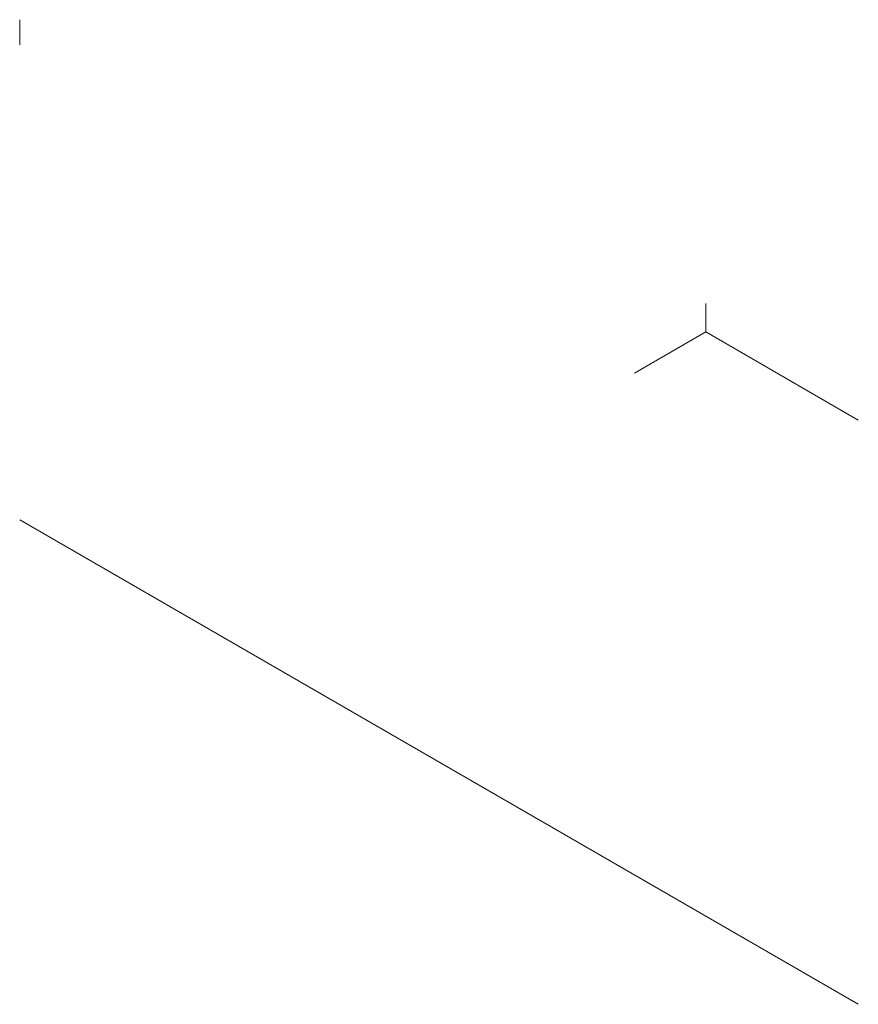
# Model space of a CAD drawing. Units: centimetres. Extents: x 97 to 8330, y -76 to 4066.
# Tile 2 of 2: x 5832 to 8330, y 1133 to 4066. Entities that reach past the tile are written whole.
import ezdxf

# ---------------------------------------------------------------- set-up
doc = ezdxf.new("R2010")
doc.units = ezdxf.units.CM
doc.header["$MEASUREMENT"] = 0
doc.layers.add('A-CONS', color=8, linetype='Continuous', lineweight=13)

msp = doc.modelspace()

# ---------------------------------------------------------------- linework, layer by layer
at = {"layer": 'A-CONS'}
for p, q in [((5831.6, 3990.6), (5831.6, 4065.6)), ((7875.5, 3135.6), (7875.5, 3220.6)), ((7663.3, 3013.1), (7875.5, 3135.6)), ((8330.1, 2873.1), (7875.5, 3135.6)), ((8330.1, 1133.1), (5831.6, 2575.6))]:
    msp.add_line(p, q, dxfattribs=at)

doc.saveas('drawing.dxf')
